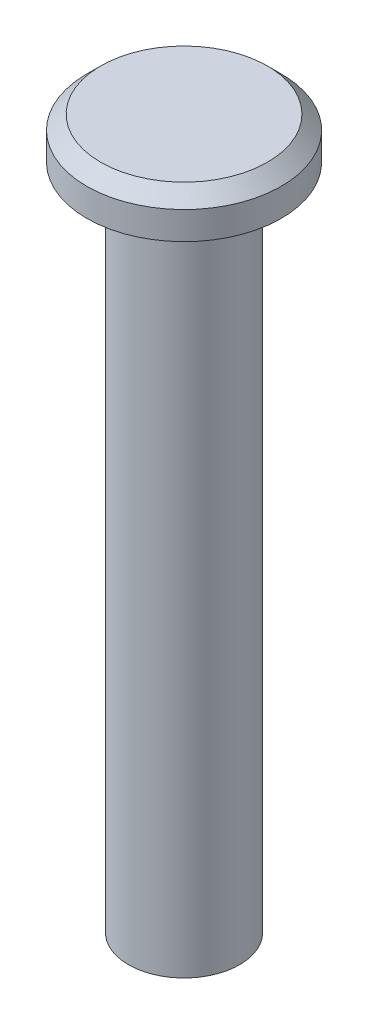
SolidWorks part; units mm, degrees
material "Plain Carbon Steel"
ref_plane "Front Plane" through (0, 0, 0) normal (0, 0, 1) x (1, 0, 0)
ref_plane "Top Plane" through (0, 0, 0) normal (0, 1, 0) x (1, 0, 0)
ref_plane "Right Plane" through (0, 0, 0) normal (1, 0, 0) x (0, 0, -1)
sketch "Shank Profile Ø8" plane through (0, 0, 0) normal (0, 1, 0) x (1, 0, 0)
  circle A0 centre (0, 0) radius 4
  dimension "D1" = 8
extrude "Shank Ø8x48" add sketch "Shank Profile Ø8" along normal blind 48
sketch "Head Profile Ø14" plane through (0, 48, 0) normal (0, 1, 0) x (1, 0, 0)
  circle A0 centre (0, 0) radius 7
  dimension "D1" = 14
extrude "Head Ø14x3" add sketch "Head Profile Ø14" along normal blind 3
chamfer "Head Chamfer 1x45°" distance 1 angle 45 1 edges at (0, 51, 7)
